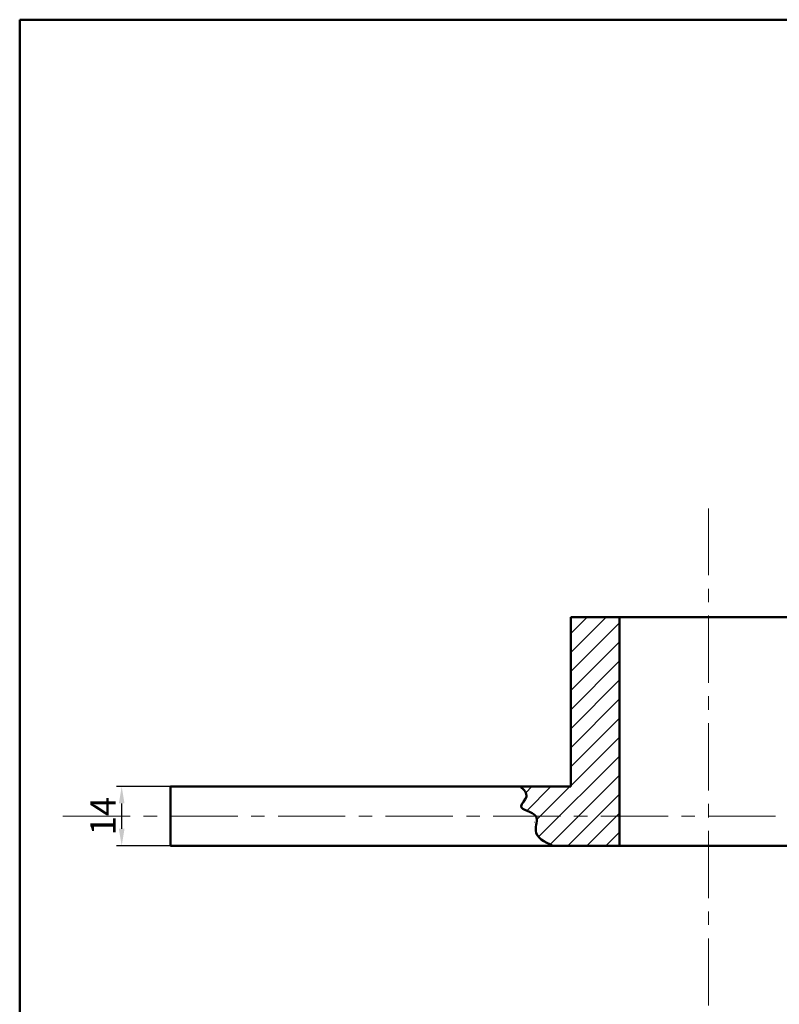
# Model space of a CAD drawing. Units: millimetres. Extents: x -1099 to -222, y 37 to 495.
# Tile 2 of 3: x -1099 to -920, y 263 to 495. Entities that reach past the tile are written whole.
import ezdxf

# ---------------------------------------------------------------- set-up
doc = ezdxf.new("R2010")
doc.units = ezdxf.units.MM
doc.header["$LTSCALE"] = 0.5
doc.linetypes.add('CENTER', pattern=[50.800000000000004, 31.75, -6.349999999999999, 6.349999999999999, -6.349999999999999])
for name, color, linetype, lineweight in [('M-CNTR', 1, 'CENTER', 18), ('M-DIMS', 2, 'Continuous', 25), ('M-HATC', 8, 'Continuous', 18), ('M-OUTL', 7, 'Continuous', 50), ('M-TTLB', 7, 'Continuous', 50)]:
    doc.layers.add(name, color=color, linetype=linetype, lineweight=lineweight)
doc.styles.get("Standard").update_dxf_attribs({"font": 'arial.ttf'})
doc.dimstyles.new('ISO-25', dxfattribs={"dimtxt": 6, "dimasz": 4, "dimexe": 1.25, "dimexo": 0.625, "dimtad": 1, "dimtoh": 1, "dimtxsty": 'Standard', "dimcen": 2.5, "dimadec": 0, "dimazin": 0, "dimtfac": 1, "dimtofl": 0, "dimtmove": 0, "dimatfit": 3, "dimfxl": 1, "dimarcsym": 0})

# ---------------------------------------------------------------- blocks, each defined once
blk = doc.blocks.new('*D19')
at = {"layer": 'Defpoints', "color": 0, "ltscale": 0.5, "transparency": 16777216}
for p in [(-1074.920599112858, 314.3451799427146), (-1042.908784497097, 314.3451799427146), (-1042.908784497097, 300.3451799427147)]:
    blk.add_point(p, dxfattribs=at)
at = {"layer": 'M-DIMS', "color": 0, "lineweight": -2, "ltscale": 0.5, "transparency": 16777216}
for p, q in [((-1043.533784497097, 314.3451799427146), (-1076.170599112858, 314.3451799427146)), ((-1074.920599112858, 304.3451799427146), (-1074.920599112858, 310.3451799427146)), ((-1043.533784497097, 300.3451799427147), (-1076.170599112858, 300.3451799427147))]:
    blk.add_line(p, q, dxfattribs=at)
at = {"layer": 'M-DIMS', "color": 0, "ltscale": 0.5, "transparency": 16777216}
for points in [[(-1075.587265779525, 310.3451799427146), (-1074.253932446191, 310.3451799427146), (-1074.920599112858, 314.3451799427146)], [(-1075.587265779525, 304.3451799427146), (-1074.253932446191, 304.3451799427146), (-1074.920599112858, 300.3451799427147)]]:
    blk.add_solid(points, dxfattribs=at)
at = {"layer": 'M-DIMS', "color": 0, "ltscale": 0.5, "transparency": 16777216, "insert": (-1078.55787742118, 307.3451799427145), "char_height": 6, "attachment_point": 5, "rotation": 90}
blk.add_mtext('14', dxfattribs=at)

msp = doc.modelspace()

# ---------------------------------------------------------------- hatches: boundary and pattern name
at = {"layer": 'M-HATC', "ltscale": 0.5}
h = msp.add_hatch(dxfattribs=at)
h.set_pattern_fill('ANSI31', color=256)
h.set_pattern_definition([(45, (-1406.913769851486, -374.9261606673909), (-2.245064030267288, 2.245064030267288), [])])
edge = h.paths.add_edge_path()
edge.add_line((-957.4196415517802, 354.3451799427145), (-968.9196415517802, 354.3451799427145))
edge.add_line((-968.9196415517802, 354.3451799427145), (-968.9196415517802, 314.3451799427146))
edge.add_line((-968.9196415517802, 314.3451799427146), (-980.812656380473, 314.3451799427146))
edge.add_spline(control_points=[(-980.812656380473, 314.3451799427146), (-980.6428850357015, 314.1812951891479), (-980.47311369093, 314.0174104355813), (-980.3125779353066, 313.8528937337513)], knot_values=[0, 0, 0, 0, 0.5848500085607816, 0.5848500085607816, 0.5848500085607816, 0.5848500085607816], degree=3, periodic=0)
edge.add_spline(control_points=[(-980.3125779353066, 313.8528937337513), (-980.1119082407918, 313.6472478564783), (-979.925669154319, 313.4406145600439), (-979.7718989359388, 313.231759570496)], knot_values=[0.5848500085607816, 0.5848500085607816, 0.5848500085607816, 0.5848500085607816, 1.315912519209611, 1.315912519209611, 1.315912519209611, 1.315912519209611], degree=3, periodic=0)
edge.add_spline(control_points=[(-979.7718989359388, 313.231759570496), (-979.7411197603025, 313.1899544376588), (-979.7116414629215, 313.1480602917935), (-979.6836087039425, 313.1060672344817)], knot_values=[1.315912519209611, 1.315912519209611, 1.315912519209611, 1.315912519209611, 1.462244505034893, 1.462244505034893, 1.462244505034893, 1.462244505034893], degree=3, periodic=0)
edge.add_spline(control_points=[(-979.6041141792057, 312.9799881768028), (-979.6290755647378, 313.0221196846876), (-979.6556217238473, 313.0641427539126), (-979.6836087039425, 313.1060672344817)], knot_values=[1.462244505034893, 1.462244505034893, 1.462244505034893, 1.462244505034893, 1.608337523479026, 1.608337523479026, 1.608337523479026, 1.608337523479026], degree=3, periodic=0)
edge.add_spline(control_points=[(-979.534384214024, 312.8537590769587), (-979.5559603849349, 312.8959495189233), (-979.5792511260069, 312.9380226408535), (-979.6041141792057, 312.9799881768028)], knot_values=[1.608337523479025, 1.608337523479025, 1.608337523479025, 1.608337523479025, 1.753855026299269, 1.753855026299269, 1.753855026299269, 1.753855026299269], degree=3, periodic=0)
edge.add_spline(control_points=[(-979.4744262277042, 312.7256099965224), (-979.492567158569, 312.7684526058259), (-979.5126019452389, 312.8111656274151), (-979.534384214024, 312.8537590769587)], knot_values=[1.753855026299269, 1.753855026299269, 1.753855026299269, 1.753855026299269, 1.900762527748943, 1.900762527748943, 1.900762527748943, 1.900762527748943], degree=3, periodic=0)
edge.add_spline(control_points=[(-979.4264044307405, 312.5984189500321), (-979.4404746229128, 312.6409485104271), (-979.4565287417558, 312.6833423199788), (-979.4744262277042, 312.7256099965224)], knot_values=[1.900762527748943, 1.900762527748943, 1.900762527748943, 1.900762527748943, 2.045698582159626, 2.045698582159626, 2.045698582159626, 2.045698582159626], degree=3, periodic=0)
edge.add_spline(control_points=[(-979.3978690646813, 312.5013881925229), (-979.406198162635, 312.5338127043666), (-979.4157304074525, 312.5661548904854), (-979.4264044307405, 312.5984189500321)], knot_values=[2.045698582159626, 2.045698582159626, 2.045698582159626, 2.045698582159626, 2.155650941096391, 2.155650941096391, 2.155650941096391, 2.155650941096391], degree=3, periodic=0)
edge.add_spline(control_points=[(-979.381605864348, 312.430395417251), (-979.3863726574469, 312.4541044445694), (-979.3918016318219, 312.4777681619133), (-979.3978690646813, 312.5013881925229)], knot_values=[2.155650941096391, 2.155650941096391, 2.155650941096391, 2.155650941096391, 2.235747076273209, 2.235747076273209, 2.235747076273209, 2.235747076273209], degree=3, periodic=0)
edge.add_spline(control_points=[(-979.3666614508094, 312.3395626174517), (-979.370535623641, 312.3699159846431), (-979.3755334423249, 312.4001924659927), (-979.381605864348, 312.430395417251)], knot_values=[2.23574707627321, 2.23574707627321, 2.23574707627321, 2.23574707627321, 2.337781615026713, 2.337781615026713, 2.337781615026713, 2.337781615026713], degree=3, periodic=0)
edge.add_spline(control_points=[(-979.3570736580589, 312.2086329430942), (-979.3574617103588, 312.2300449669449), (-979.358435082815, 312.2514169400689), (-979.3599769405266, 312.2727500143999)], knot_values=[2.412506285213873, 2.412506285213873, 2.412506285213873, 2.412506285213873, 2.483949308450005, 2.483949308450005, 2.483949308450005, 2.483949308450005], degree=3, periodic=0)
edge.add_spline(control_points=[(-979.3577978801991, 312.1412730565519), (-979.3569025125059, 312.1637710995183), (-979.356667537672, 312.1862239548832), (-979.3570736580589, 312.2086329430942)], knot_values=[2.483949308450005, 2.483949308450005, 2.483949308450005, 2.483949308450005, 2.558718787347598, 2.558718787347598, 2.558718787347598, 2.558718787347598], degree=3, periodic=0)
edge.add_spline(control_points=[(-979.3707709583157, 312.0087593085831), (-979.3672170936618, 312.0314512114263), (-979.3643621025413, 312.0540952936152), (-979.3621866564622, 312.0766928777083)], knot_values=[2.630121983330612, 2.630121983330612, 2.630121983330612, 2.630121983330612, 2.704931289482556, 2.704931289482556, 2.704931289482556, 2.704931289482556], degree=3, periodic=0)
edge.add_spline(control_points=[(-979.3828669676194, 311.9436838377156), (-979.3781877299679, 311.9654199485779), (-979.3741613207375, 311.9871113894378), (-979.3707709583157, 312.0087593085831)], knot_values=[2.704931289482557, 2.704931289482557, 2.704931289482557, 2.704931289482557, 2.77629885270907, 2.77629885270907, 2.77629885270907, 2.77629885270907], degree=3, periodic=0)
edge.add_spline(control_points=[(-979.4310818138583, 311.7773436827926), (-979.4191772567177, 311.8103077297813), (-979.4086123854094, 311.843195627723), (-979.3995297510445, 311.875984122095)], knot_values=[2.850234410940849, 2.850234410940849, 2.850234410940849, 2.850234410940849, 2.957430435272468, 2.957430435272468, 2.957430435272468, 2.957430435272468], degree=3, periodic=0)
edge.add_spline(control_points=[(-979.4723657489662, 311.6743772643608), (-979.4572648865905, 311.7087642164905), (-979.4434502834403, 311.7430950494615), (-979.4310818138583, 311.7773436827926)], knot_values=[2.957430435272467, 2.957430435272467, 2.957430435272467, 2.957430435272467, 3.068803815281008, 3.068803815281008, 3.068803815281008, 3.068803815281008], degree=3, periodic=0)
edge.add_spline(control_points=[(-979.5359486771443, 311.54285486845), (-979.5128903642982, 311.5867507301083), (-979.4915861692734, 311.6306094545117), (-979.4723657489662, 311.6743772643608)], knot_values=[3.068803815281008, 3.068803815281008, 3.068803815281008, 3.068803815281008, 3.2105601680996, 3.2105601680996, 3.2105601680996, 3.2105601680996], degree=3, periodic=0)
edge.add_spline(control_points=[(-979.6145166486157, 311.4036666590392), (-979.5866285738679, 311.4500619031929), (-979.560309668485, 311.4964791117817), (-979.5359486771443, 311.54285486845)], knot_values=[3.2105601680996, 3.2105601680996, 3.2105601680996, 3.2105601680996, 3.360325040598847, 3.360325040598847, 3.360325040598847, 3.360325040598847], degree=3, periodic=0)
edge.add_spline(control_points=[(-979.6145166486157, 311.4036666590392), (-979.7620536893209, 311.1582206364237), (-979.9535079549153, 310.9133893447962), (-980.1313206019225, 310.6785624229087)], knot_values=[3.360325040598847, 3.360325040598847, 3.360325040598847, 3.360325040598847, 4.152630220858404, 4.152630220858404, 4.152630220858404, 4.152630220858404], degree=3, periodic=0)
edge.add_spline(control_points=[(-980.1313206019225, 310.6785624229087), (-980.2829155758608, 310.4783596718519), (-980.4245951503709, 310.2854285888426), (-980.5206913445177, 310.105587731652)], knot_values=[4.152630220858404, 4.152630220858404, 4.152630220858404, 4.152630220858404, 4.828113574681904, 4.828113574681904, 4.828113574681904, 4.828113574681904], degree=3, periodic=0)
edge.add_spline(control_points=[(-980.5206913445177, 310.105587731652), (-980.5354658029187, 310.0779378201547), (-980.549162761288, 310.0505973354401), (-980.5616525928644, 310.0235874236675)], knot_values=[4.828113574681904, 4.828113574681904, 4.828113574681904, 4.828113574681904, 4.931966810497659, 4.931966810497659, 4.931966810497659, 4.931966810497659], degree=3, periodic=0)
edge.add_spline(control_points=[(-980.5616525928644, 310.0235874236675), (-980.5718586544285, 310.0015162835794), (-980.5812586769233, 309.9796658781382), (-980.5897819310298, 309.9580477454972)], knot_values=[4.931966810497659, 4.931966810497659, 4.931966810497659, 4.931966810497659, 5.016830446320926, 5.016830446320926, 5.016830446320926, 5.016830446320926], degree=3, periodic=0)
edge.add_spline(control_points=[(-980.5897819310298, 309.9580477454972), (-980.5996992228957, 309.9328938162215), (-980.6084294888487, 309.9080543529282), (-980.6158613090694, 309.8835475316576)], knot_values=[5.016830446320926, 5.016830446320926, 5.016830446320926, 5.016830446320926, 5.115574122706974, 5.115574122706974, 5.115574122706974, 5.115574122706974], degree=3, periodic=0)
edge.add_spline(control_points=[(-980.6158613090694, 309.8835475316576), (-980.6212812668094, 309.8656749336017), (-980.6260106267135, 309.8479792561944), (-980.6300061707913, 309.8304675496349)], knot_values=[5.115574122706974, 5.115574122706974, 5.115574122706974, 5.115574122706974, 5.187586972480812, 5.187586972480812, 5.187586972480812, 5.187586972480812], degree=3, periodic=0)
edge.add_spline(control_points=[(-980.6300061707913, 309.8304675496349), (-980.6341228133311, 309.8124250916447), (-980.6374604844277, 309.7945779252137), (-980.6399719161859, 309.7769337612066)], knot_values=[5.187586972480812, 5.187586972480812, 5.187586972480812, 5.187586972480812, 5.261782414962654, 5.261782414962654, 5.261782414962654, 5.261782414962654], degree=3, periodic=0)
edge.add_spline(control_points=[(-980.6399719161859, 309.7769337612066), (-980.6423770932553, 309.7600360937539), (-980.6440355019249, 309.743212660305), (-980.6448838417738, 309.7265847822722), (-980.6448894513279, 309.7264741379121)], knot_values=[5.261782414962654, 5.261782414962654, 5.261782414962654, 5.261782414962654, 5.332838766119513, 5.33331479037324, 5.33331479037324, 5.33331479037324, 5.33331479037324], degree=3, periodic=0)
edge.add_spline(control_points=[(-980.6448894513279, 309.7264741379121), (-980.6455466742706, 309.7135108946627), (-980.6457115634877, 309.7006664972992), (-980.6453952735285, 309.6879375038484)], knot_values=[5.33331479037324, 5.33331479037324, 5.33331479037324, 5.33331479037324, 5.389086437343398, 5.389086437343398, 5.389086437343398, 5.389086437343398], degree=3, periodic=0)
edge.add_spline(control_points=[(-980.6453952735285, 309.6879375038484), (-980.644777689205, 309.6630830100956), (-980.6423255591534, 309.6386685057808), (-980.6381219228526, 309.614668367311)], knot_values=[5.389086437343398, 5.389086437343398, 5.389086437343398, 5.389086437343398, 5.497985546810505, 5.497985546810505, 5.497985546810505, 5.497985546810505], degree=3, periodic=0)
edge.add_spline(control_points=[(-980.6381219228526, 309.614668367311), (-980.6359693311794, 309.6023784129648), (-980.6333574518902, 309.5901971154396), (-980.6302974354807, 309.5781210340136)], knot_values=[5.497985546810505, 5.497985546810505, 5.497985546810505, 5.497985546810505, 5.55375043689149, 5.55375043689149, 5.55375043689149, 5.55375043689149], degree=3, periodic=0)
edge.add_spline(control_points=[(-980.6302974354807, 309.5781210340136), (-980.6263656253531, 309.5626044965515), (-980.6216939570413, 309.5472616670651), (-980.6163060843239, 309.5320852466792)], knot_values=[5.55375043689149, 5.55375043689149, 5.55375043689149, 5.55375043689149, 5.625402653821721, 5.625402653821721, 5.625402653821721, 5.625402653821721], degree=3, periodic=0)
edge.add_spline(control_points=[(-980.6163060843239, 309.5320852466792), (-980.6107047679983, 309.5163076038634), (-980.6043293775803, 309.5007098160896), (-980.5972064908583, 309.4852836822172)], knot_values=[5.625402653821721, 5.625402653821721, 5.625402653821721, 5.625402653821721, 5.699893413627985, 5.699893413627985, 5.699893413627985, 5.699893413627985], degree=3, periodic=0)
edge.add_spline(control_points=[(-980.5972064908583, 309.4852836822172), (-980.5903486660902, 309.4704315966688), (-980.5827979426297, 309.4557386273105), (-980.5745780402142, 309.4411974549137)], knot_values=[5.699893413627985, 5.699893413627985, 5.699893413627985, 5.699893413627985, 5.77161217001588, 5.77161217001588, 5.77161217001588, 5.77161217001588], degree=3, periodic=0)
edge.add_spline(control_points=[(-980.5745780402142, 309.4411974549137), (-980.5660494352911, 309.4261101815837), (-980.5568004448986, 309.4111863209322), (-980.5468575628141, 309.3964176977423)], knot_values=[5.77161217001588, 5.77161217001588, 5.77161217001588, 5.77161217001588, 5.846024359831157, 5.846024359831157, 5.846024359831157, 5.846024359831157], degree=3, periodic=0)
edge.add_spline(control_points=[(-980.5468575628141, 309.3964176977423), (-980.5372640347186, 309.38216798621), (-980.5270245195712, 309.3680627949124), (-980.5161628154603, 309.3540947804442)], knot_values=[5.846024359831157, 5.846024359831157, 5.846024359831157, 5.846024359831157, 5.917821996328149, 5.917821996328149, 5.917821996328149, 5.917821996328149], degree=3, periodic=0)
edge.add_spline(control_points=[(-980.5161628154603, 309.3540947804442), (-980.5049198488229, 309.3396364671766), (-980.4930102470317, 309.3253251299921), (-980.4804604032192, 309.3111526247298)], knot_values=[5.917821996328149, 5.917821996328149, 5.917821996328149, 5.917821996328149, 5.992139840336784, 5.992139840336784, 5.992139840336784, 5.992139840336784], degree=3, periodic=0)
edge.add_spline(control_points=[(-980.4804604032192, 309.3111526247298), (-980.462387113411, 309.2907425065848), (-980.4429859951866, 309.2706203185744), (-980.4223358778354, 309.250761736249)], knot_values=[5.992139840336784, 5.992139840336784, 5.992139840336784, 5.992139840336784, 6.099166505589271, 6.099166505589271, 6.099166505589271, 6.099166505589271], degree=3, periodic=0)
edge.add_spline(control_points=[(-980.4223358778354, 309.250761736249), (-980.4077963728905, 309.2367795418136), (-980.3926376887927, 309.2229280273291), (-980.3768873405025, 309.2091987024709)], knot_values=[6.099166505589271, 6.099166505589271, 6.099166505589271, 6.099166505589271, 6.174522722806481, 6.174522722806481, 6.174522722806481, 6.174522722806481], degree=3, periodic=0)
edge.add_spline(control_points=[(-980.3768873405025, 309.2091987024709), (-980.3542917332832, 309.1895024756848), (-980.3304784185211, 309.1700577280847), (-980.3055286363184, 309.1508393913135)], knot_values=[6.174522722806481, 6.174522722806481, 6.174522722806481, 6.174522722806481, 6.282629505869842, 6.282629505869842, 6.282629505869842, 6.282629505869842], degree=3, periodic=0)
edge.add_spline(control_points=[(-980.3055286363184, 309.1508393913135), (-980.2716191482298, 309.1247195656359), (-980.235610401511, 309.0990179612548), (-980.1977063509413, 309.0736716435961)], knot_values=[6.282629505869842, 6.282629505869842, 6.282629505869842, 6.282629505869842, 6.429558470732539, 6.429558470732539, 6.429558470732539, 6.429558470732539], degree=3, periodic=0)
edge.add_spline(control_points=[(-980.1977063509413, 309.0736716435961), (-980.1554009807949, 309.0453821775819), (-980.1107345964551, 309.0175352986462), (-980.063990770032, 308.9900435045983)], knot_values=[6.429558470732539, 6.429558470732539, 6.429558470732539, 6.429558470732539, 6.593548444107618, 6.593548444107618, 6.593548444107618, 6.593548444107618], degree=3, periodic=0)
edge.add_spline(control_points=[(-980.063990770032, 308.9900435045983), (-980.0065399611835, 308.9562545333991), (-979.9459510095593, 308.9230019463833), (-979.8827503918843, 308.8901232879881)], knot_values=[6.593548444107618, 6.593548444107618, 6.593548444107618, 6.593548444107618, 6.795101404881557, 6.795101404881557, 6.795101404881557, 6.795101404881557], degree=3, periodic=0)
edge.add_spline(control_points=[(-979.8827503918843, 308.8901232879881), (-979.7917466660649, 308.8427807061593), (-979.6953280040366, 308.7962134147344), (-979.5950661893066, 308.7499364065657)], knot_values=[6.795101404881557, 6.795101404881557, 6.795101404881557, 6.795101404881557, 7.085321201065431, 7.085321201065431, 7.085321201065431, 7.085321201065431], degree=3, periodic=0)
edge.add_spline(control_points=[(-979.5950661893066, 308.7499364065657), (-979.3330390858162, 308.6289947455625), (-979.044763212723, 308.5100357219682), (-978.7582945015321, 308.3844020828949)], knot_values=[7.085321201065431, 7.085321201065431, 7.085321201065431, 7.085321201065431, 7.843789943870335, 7.843789943870335, 7.843789943870335, 7.843789943870335], degree=3, periodic=0)
edge.add_spline(control_points=[(-978.7582945015321, 308.3844020828949), (-978.665362882632, 308.3436460177077), (-978.5726214458497, 308.3021875292861), (-978.4810280105617, 308.2597310621411)], knot_values=[7.843789943870335, 7.843789943870335, 7.843789943870335, 7.843789943870335, 8.089840299111705, 8.089840299111705, 8.089840299111705, 8.089840299111705], degree=3, periodic=0)
edge.add_spline(control_points=[(-978.4810280105617, 308.2597310621411), (-978.3321911301566, 308.1907404395817), (-978.1863855913197, 308.1191146162809), (-978.0477212088412, 308.0435854216932)], knot_values=[8.089840299111705, 8.089840299111705, 8.089840299111705, 8.089840299111705, 8.489665539659123, 8.489665539659123, 8.489665539659123, 8.489665539659123], degree=3, periodic=0)
edge.add_spline(control_points=[(-978.0477212088412, 308.0435854216932), (-977.9765063708527, 308.0047953642911), (-977.9071750938209, 307.9649757484552), (-977.8402841004805, 307.9239547855746)], knot_values=[8.489665539659123, 8.489665539659123, 8.489665539659123, 8.489665539659123, 8.695006588459075, 8.695006588459075, 8.695006588459075, 8.695006588459075], degree=3, periodic=0)
edge.add_spline(control_points=[(-977.8402841004805, 307.9239547855746), (-977.7777550742697, 307.8856088030282), (-977.7173584465057, 307.8462130447606), (-977.659548975888, 307.8056271853271)], knot_values=[8.695006588459075, 8.695006588459075, 8.695006588459075, 8.695006588459075, 8.886957330724037, 8.886957330724037, 8.886957330724037, 8.886957330724037], degree=3, periodic=0)
edge.add_spline(control_points=[(-977.659548975888, 307.8056271853271), (-977.6070150523766, 307.7687450894984), (-977.556617636746, 307.7308801927125), (-977.5086980032703, 307.691927187552)], knot_values=[8.886957330724037, 8.886957330724037, 8.886957330724037, 8.886957330724037, 9.061391130313895, 9.061391130313895, 9.061391130313895, 9.061391130313895], degree=3, periodic=0)
edge.add_spline(control_points=[(-977.3938946489575, 307.591875604883), (-977.4302972427452, 307.6260278587766), (-977.4686315219733, 307.6593578680574), (-977.5086980032703, 307.691927187552)], knot_values=[9.061391130313893, 9.061391130313893, 9.061391130313893, 9.061391130313893, 9.207238417989698, 9.207238417989698, 9.207238417989698, 9.207238417989698], degree=3, periodic=0)
edge.add_spline(control_points=[(-977.2901929898424, 307.4863487502941), (-977.32267401134, 307.5223965750947), (-977.3573087351492, 307.5575513634676), (-977.3938946489575, 307.591875604883)], knot_values=[9.207238417989698, 9.207238417989698, 9.207238417989698, 9.207238417989698, 9.35382017881778, 9.35382017881778, 9.35382017881778, 9.35382017881778], degree=3, periodic=0)
edge.add_spline(control_points=[(-977.2218761025163, 307.4050490684093), (-977.2434209638319, 307.4326521624783), (-977.2662203981241, 307.4597436822748), (-977.2901929898424, 307.4863487502941)], knot_values=[9.35382017881778, 9.35382017881778, 9.35382017881778, 9.35382017881778, 9.462004729169475, 9.462004729169475, 9.462004729169475, 9.462004729169475], degree=3, periodic=0)
edge.add_line((-977.1733550786192, 307.3451799427145), (-957.4196415517802, 307.3451799427145))
edge.add_line((-957.4196415517802, 307.3451799427145), (-957.4196415517802, 354.3451799427145))
edge = h.paths.add_edge_path()
edge.add_line((-957.4196415517802, 307.3451799427145), (-977.1777089217263, 307.3451799427145))
edge.add_spline(control_points=[(-977.1777089217263, 307.3451799427144), (-976.5558447964703, 306.4509998490912), (-978.3221876801773, 302.7832358604618), (-975.1132695777359, 301.2713065293687), (-973.1476589450494, 300.3451799427145)], knot_values=[9.539187125630672, 9.539187125630688, 9.539187125630688, 9.539187125630688, 12.95191047053349, 18.34726556679153, 18.34726556679153, 18.34726556679153, 18.34726556679153], degree=3, periodic=0)
edge.add_line((-973.1476589450496, 300.3451799427145), (-957.4196415517802, 300.3451799427145))
edge.add_line((-957.4196415517802, 300.3451799427145), (-957.4196415517802, 307.3451799427145))

# ---------------------------------------------------------------- linework, layer by layer
at = {"layer": 'M-CNTR'}
for p, q in [((-936.41964155178, 135.6015347866727), (-936.41964155178, 379.9691777230995)), ((-1088.8088415032, 307.3451799427145), (-798.9646638206668, 307.3451799427145))]:
    msp.add_line(p, q, dxfattribs=at)
at = {"layer": 'M-OUTL'}
for p, q in [((-968.9196415517802, 354.3451799427145), (-903.91964155178, 354.3451799427145)), ((-968.9196415517802, 314.3451799427146), (-968.9196415517802, 354.3451799427146)), ((-957.4196415517802, 300.3451799427145), (-957.4196415517802, 354.3451799427145)), ((-1063.41964155178, 314.3451799427146), (-968.9196415517802, 314.3451799427146)), ((-1063.41964155178, 314.3451799427146), (-1063.41964155178, 300.3451799427145)), ((-1063.41964155178, 300.3451799427145), (-825.41964155178, 300.3451799427145))]:
    msp.add_line(p, q, dxfattribs=at)
at = {"layer": 'M-OUTL', "ltscale": 0.5}
msp.add_open_spline([(-980.812656380473, 314.3451799427146), (-979.9899386070167, 313.5509887926165), (-978.4419122831364, 312.0566381827111), (-982.3291444707443, 308.9281398888047), (-975.7123176252665, 308.2025615704935), (-978.3221876801773, 302.7832358604618), (-975.1132695777359, 301.2713065293687), (-973.1476589450494, 300.3451799427145)], degree=3, knots=[0, 0, 0, 0, 2.834203248473524, 5.332838766119513, 9.539187125630672, 12.95191047053349, 18.34726556679153, 18.34726556679153, 18.34726556679153, 18.34726556679153], dxfattribs=at)
at = {"layer": 'M-TTLB', "ltscale": 0.5}
msp.add_lwpolyline([(-1099.004687419986, 495.3704252679146), (-222.2054647419409, 495.3704252679146), (-222.2054647419409, 36.58144759589982), (-1099.004687419986, 36.58144759589982)], close=True, dxfattribs=at)

# ---------------------------------------------------------------- dimensions: what is measured, and where the dimension line sits
at = {"layer": 'M-DIMS', "ltscale": 0.5}
dim = msp.add_linear_dim(base=(-1074.920599112858, 314.3451799427146), p1=(-1042.908784497096, 300.3451799427145), p2=(-1042.908784497096, 314.3451799427146), angle=90, dimstyle='ISO-25', override={"dimclrd": 0, "dimclre": 0, "dimclrt": 0}, dxfattribs=at)
dim.commit()
dim.dimension.update_dxf_attribs({"geometry": '*D19', "text_midpoint": (-1074.920599112858, 307.3451799427145), "dimtype": 160})

doc.saveas('drawing.dxf')
